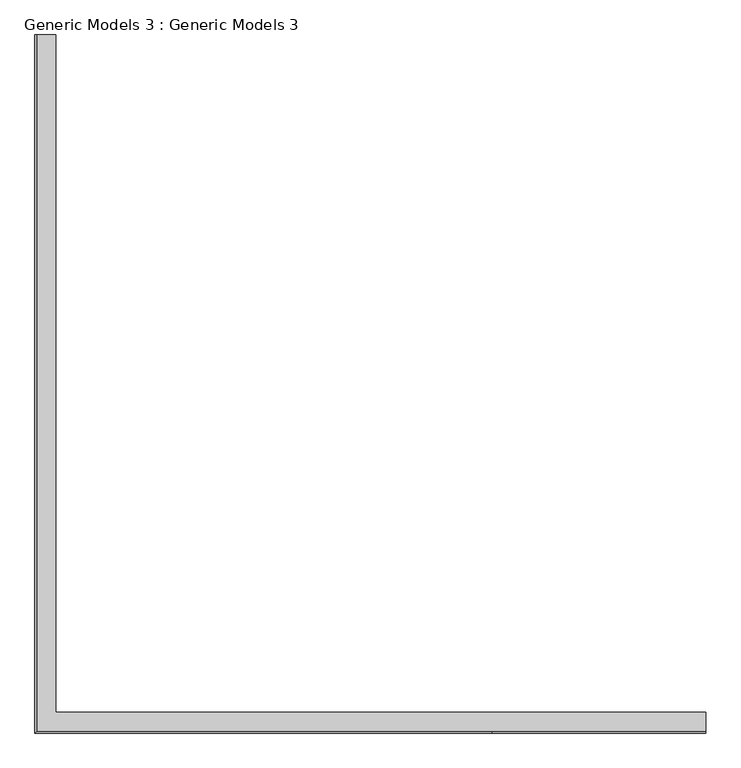
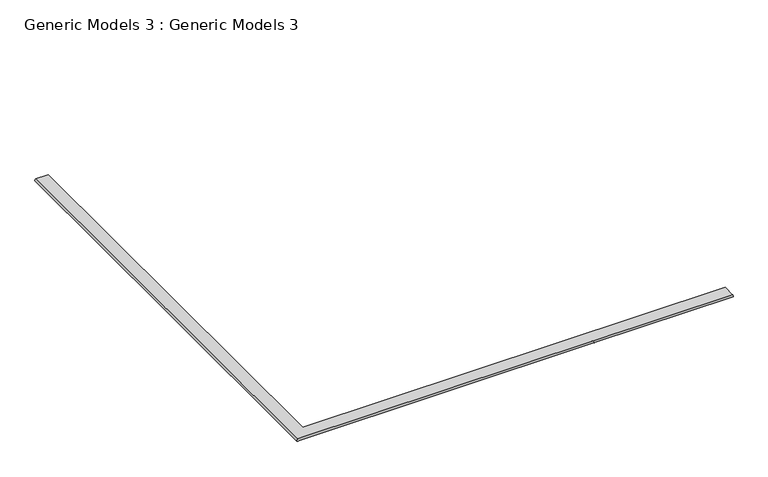
"""IFC4 building model written with IfcOpenShell, lengths in millimetres: proxy geometry, Generic Models 3 : Generic Models 3."""

from ifc_helpers import new_model, si_unit, frame, origin, place, context, project, spatial, circle_curve, ellipse_curve, source, transform, mapped, element, save
from ifc_brep_helpers import plane_surface, cylinder_surface, advanced_brep


def generic_models_3_generic_models_3_cf0a2ed0(model_context):
    return source(origin(), model_context, "Body", "AdvancedBrep", [
        advanced_brep(
        [(-8026.7525595, 1694.8132107, 6858.0), (-8026.7525595, 1694.8132107, 6883.4), (-7880.7025595, 1694.8132107, 6883.4), (-7880.7025595, 1694.8132107, 6858.0), (-8026.7525595, -3632.8367893, 6858.0), (-8026.7525595, -3632.8367893, 6883.4), (-4546.9525595, -3632.8367893, 6883.4), (-2906.3946608, -3632.8367893, 6883.4), (-2906.3946608, -3486.7867893, 6883.4), (-7880.7025595, -3486.7867893, 6883.4), (-7880.7025595, -3486.7867893, 6858.0), (-2906.3946608, -3486.7867893, 6858.0), (-2906.3946608, -3632.8367893, 6858.0), (-4546.9525595, -3632.8367893, 6858.0)],
        [
            (0, 1, circle_curve(frame((-8026.7525595, 1694.8132107, 6870.7), z_axis=(0.0, 1.0, 0.0), x_axis=(1.0, 0.0, 0.0)), 12.7)),
            (1, 2),
            (2, 3),
            (3, 0),
            (0, 4),
            (4, 5, ellipse_curve(frame((-8026.7525595, -3632.8367893, 6870.7), z_axis=(-0.7071067811865475, 0.7071067811865475, 0.0), x_axis=(0.7071067811865474, 0.7071067811865476, 0.0)), 17.9605122, 12.7)),
            (5, 1),
            (5, 6),
            (6, 7),
            (7, 8),
            (8, 9),
            (9, 2),
            (9, 10),
            (10, 3),
            (10, 11),
            (11, 12),
            (12, 13),
            (13, 4),
            (13, 6, circle_curve(frame((-4546.9525595, -3632.8367893, 6870.7), z_axis=(-1.0, 0.0, 0.0), x_axis=(0.0, 1.0, 0.0)), 12.7)),
            (8, 11),
            (7, 12, circle_curve(frame((-2906.3946608, -3632.8367893, 6870.7), z_axis=(1.0, 0.0, 0.0), x_axis=(0.0, 1.0, 0.0)), 12.7)),
        ],
        [
            plane_surface(frame((-7937.8525595, 1694.8132107, 6858.0), z_axis=(0.0, 1.0, 0.0), x_axis=(0.0, 0.0, 1.0))),
            cylinder_surface(frame((-8026.7525595, 1694.8132107, 6870.7), z_axis=(0.0, 1.0, 0.0), x_axis=(1.0, 0.0, 0.0)), 12.7),
            plane_surface(frame((-8026.7525595, 1694.8132107, 6883.4), z_axis=(0.0, 0.0, 1.0), x_axis=(0.0, -1.0, 0.0))),
            plane_surface(frame((-7880.7025595, 1694.8132107, 6883.4), z_axis=(1.0, 0.0, 0.0), x_axis=(0.0, -1.0, 0.0))),
            plane_surface(frame((-7880.7025595, 1694.8132107, 6858.0), z_axis=(0.0, 0.0, -1.0), x_axis=(0.0, -1.0, 0.0))),
            cylinder_surface(frame((-7937.8525595, -3632.8367893, 6870.7), z_axis=(-1.0, 0.0, 0.0), x_axis=(0.0, 1.0, 0.0)), 12.7),
            plane_surface(frame((-7880.7025595, -3486.7867893, 6883.4), z_axis=(0.0, 1.0, 0.0), x_axis=(1.0, 0.0, 0.0))),
            plane_surface(frame((-2906.3946608, -3543.9367893, 6858.0), z_axis=(1.0, 0.0, 0.0), x_axis=(0.0, 0.0, 1.0))),
            cylinder_surface(frame((-4546.9525595, -3632.8367893, 6870.7), z_axis=(-1.0, 0.0, 0.0), x_axis=(0.0, 1.0, 0.0)), 12.7),
        ],
        [
            (0, [[1, 2, 3, 4]]),
            (1, [[-1, 5, 6, 7]]),
            (2, [[-2, -7, 8, 9, 10, 11, 12]]),
            (3, [[-3, -12, 13, 14]]),
            (4, [[-4, -14, 15, 16, 17, 18, -5]]),
            (5, [[-6, -18, 19, -8]]),
            (6, [[-15, -13, -11, 20]]),
            (7, [[-16, -20, -10, 21]]),
            (8, [[-19, -17, -21, -9]]),
        ],
    ),
    ])


if __name__ == "__main__":
    model = new_model("IFC4")
    model_context = context("Model", 3, world=origin())
    ifc_project = project(units=[si_unit("LENGTHUNIT", "METRE", prefix="MILLI")], contexts=[model_context])
    site = spatial("IfcSite", under=ifc_project)
    building = spatial("IfcBuilding", under=site)
    placement = place(None, origin())
    generic_models_3_generic_models_3_shape = generic_models_3_generic_models_3_cf0a2ed0(model_context)
    element("IfcBuildingElementProxy", 1, Name="Generic Models 3 : Generic Models 3", ObjectType="Generic Models 3 : Generic Models 3", at=placement, inside=building, context=model_context, shape_type="MappedRepresentation", body=[
        mapped(generic_models_3_generic_models_3_shape, transform((0.0, 0.0, 0.0), x_axis=(1.0, 0.0, 0.0), y_axis=(0.0, 1.0, 0.0), z_axis=(0.0, 0.0, 1.0))),
    ])
    save(model, "model.ifc")
